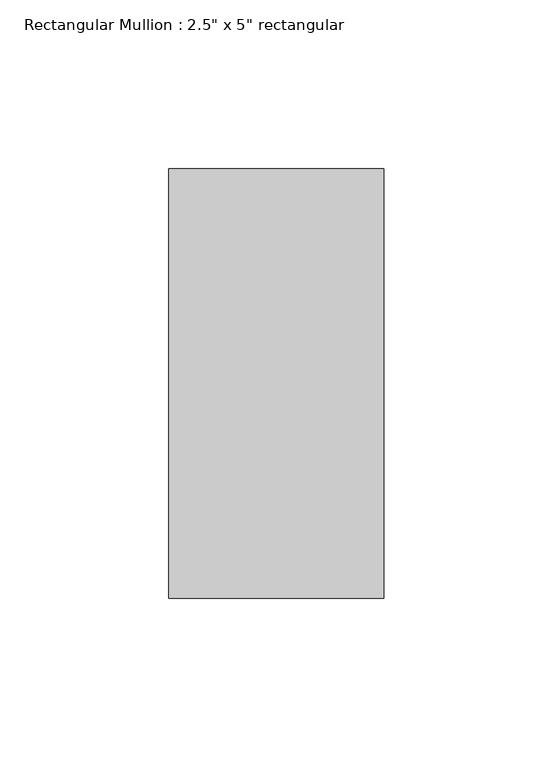
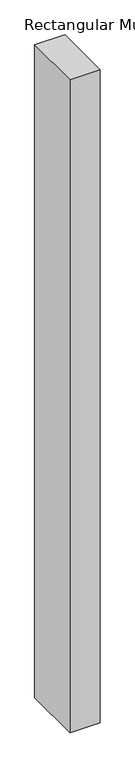
"""IFC4 building model written with IfcOpenShell, lengths in millimetres: member geometry."""

from ifc_helpers import new_model, si_unit, frame, origin, place, context, project, spatial, polyline, outline, extrude, source, transform, mapped, element, save


def member_25243d18(model_context):
    return source(origin(), model_context, "Body", "SweptSolid", [
        extrude(outline(polyline([(31.75, 63.5), (31.75, -63.5), (-31.75, -63.5), (-31.75, 63.5), (31.75, 63.5)])), frame((0.0, 0.0, -1441.7145247), z_axis=(0.0, 0.0, 1.0), x_axis=(1.0, 0.0, 0.0)), (0.0, 0.0, 1.0), 1441.7145247),
    ])


if __name__ == "__main__":
    model = new_model("IFC4")
    model_context = context("Model", 3, world=origin())
    ifc_project = project(units=[si_unit("LENGTHUNIT", "METRE", prefix="MILLI")], contexts=[model_context])
    site = spatial("IfcSite", under=ifc_project)
    building = spatial("IfcBuilding", under=site)
    placement = place(None, origin())
    member_shape = member_25243d18(model_context)
    element("IfcMember", 1, ObjectType="Rectangular Mullion : 2.5\" x 5\" rectangular", at=placement, inside=building, context=model_context, shape_type="MappedRepresentation", body=[
        mapped(member_shape, transform((0.0, 0.0, 0.0), x_axis=(1.0, 0.0, 0.0), y_axis=(0.0, 1.0, 0.0), z_axis=(0.0, 0.0, 1.0))),
    ])
    save(model, "model.ifc")

# Revit data of these elements
# Type "Rectangular Mullion : 2.5\" x 5\" rectangular"
#   built-in parameter 1007304 = 0.416667 (stored number, unit not read)
#   built-in parameter 1007301 = 0.104167 (stored number, unit not read)
#   built-in parameter 1007300 = 0.104167 (stored number, unit not read)
# Element 1 (IfcMember, "Rectangular Mullion : 2.5\" x 5\" rectangular")
#   Materials on its faces: "Aluminum"
# Materials
#   "Aluminum": class "Metal", colour RGB 247 247 247, transparency 0, Description = "Aluminum 6061", Cost = 0
